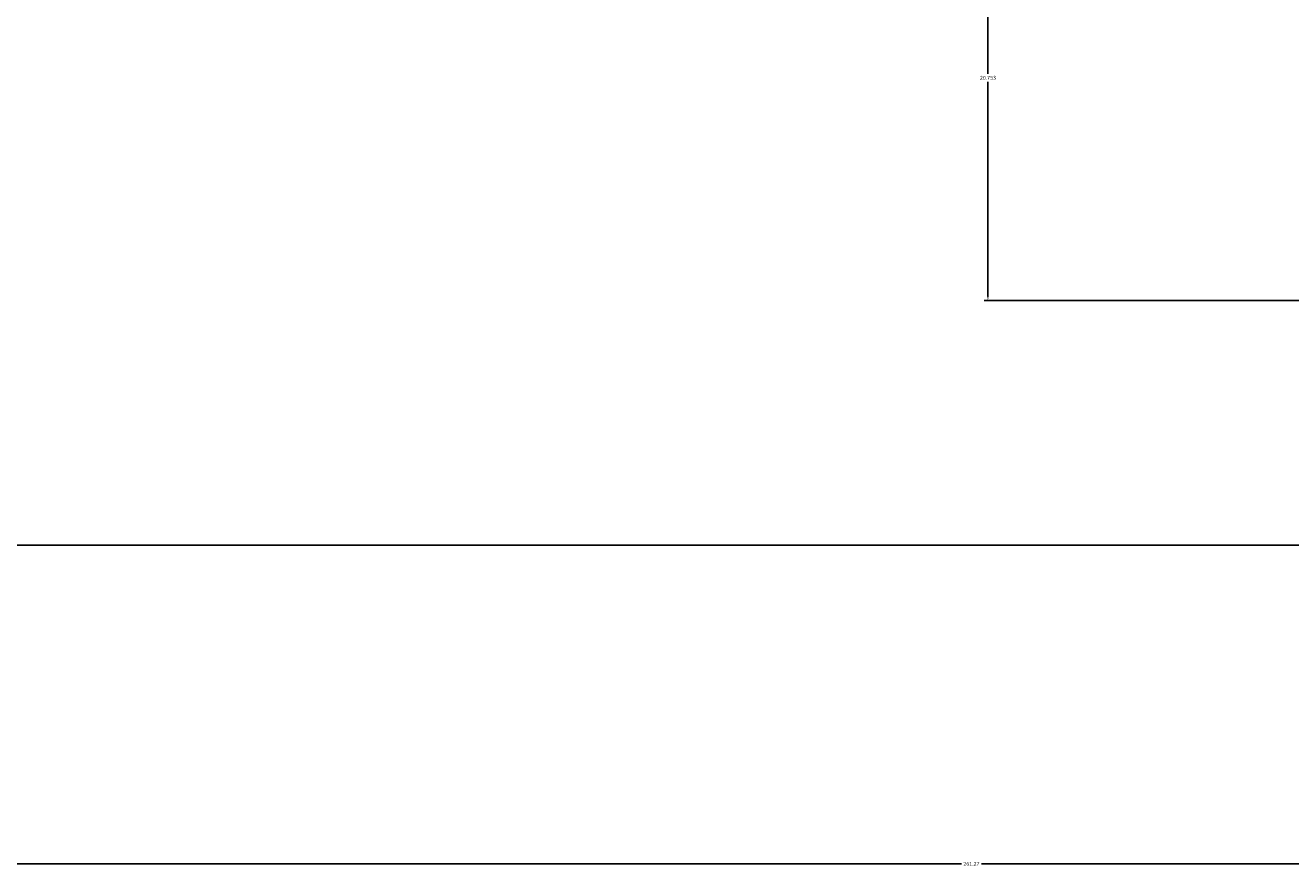
# Model space of a CAD drawing. Units: millimetres. Extents: x -11 to 280, y -4 to 208.
# Tile 19 of 55: x 91 to 150, y -4 to 36. Entities that reach past the tile are written whole.
import ezdxf

# ---------------------------------------------------------------- set-up
doc = ezdxf.new("R2010")
doc.units = ezdxf.units.MM
doc.layers.add('M-DIMS', color=2, linetype='Continuous', lineweight=18)
doc.styles.get("Standard").update_dxf_attribs({"font": 'arial.ttf'})
doc.dimstyles.get("Standard").update_dxf_attribs({"dimtxt": 0.18, "dimasz": 0.18, "dimexe": 0.18, "dimexo": 0.0625, "dimgap": 0.09, "dimtad": 0, "dimtih": 1, "dimtoh": 1, "dimdec": 4, "dimzin": 0, "dimdsep": 46, "dimtxsty": 'Standard', "dimcen": 0.09, "dimadec": 0, "dimazin": 0, "dimtfac": 1, "dimtdec": 4, "dimtofl": 0, "dimtmove": 0, "dimatfit": 3, "dimfxl": 1, "dimtolj": 1, "dimtzin": 0, "dimarcsym": 0})

# ---------------------------------------------------------------- blocks, each defined once
blk = doc.blocks.new('*D4')
at = {"layer": 'Defpoints', "color": 0, "transparency": 16777216}
for p in [(4.763, 84.426), (266.035, 51.733), (266.035, -3.415)]:
    blk.add_point(p, dxfattribs=at)
at = {"layer": 'M-DIMS', "color": 0, "lineweight": -2, "transparency": 16777216}
for p, q in [((4.763, 84.364), (4.763, -3.595)), ((266.035, 51.67), (266.035, -3.595)), ((4.943, -3.415), (134.934, -3.415)), ((265.855, -3.415), (135.864, -3.415))]:
    blk.add_line(p, q, dxfattribs=at)
at = {"layer": 'M-DIMS', "color": 0, "transparency": 16777216}
for points in [[(4.943, -3.385), (4.943, -3.445), (4.763, -3.415)], [(265.855, -3.385), (265.855, -3.445), (266.035, -3.415)]]:
    blk.add_solid(points, dxfattribs=at)
at = {"layer": 'M-DIMS', "color": 0, "transparency": 16777216, "insert": (135.399, -3.415), "char_height": 0.18, "attachment_point": 5}
blk.add_mtext('\\A1;261.27', dxfattribs=at)
blk = doc.blocks.new('*D5')
at = {"layer": 'Defpoints', "color": 0, "transparency": 16777216}
for p in [(24.759, 192.645), (-10.087, 11.435), (261.686, 11.435)]:
    blk.add_point(p, dxfattribs=at)
at = {"layer": 'M-DIMS', "color": 0, "lineweight": -2, "transparency": 16777216}
for p, q in [((24.696, 192.645), (-10.267, 192.645)), ((-10.087, 192.465), (-10.087, 102.222)), ((-10.087, 11.615), (-10.087, 101.858)), ((261.624, 11.435), (-10.267, 11.435))]:
    blk.add_line(p, q, dxfattribs=at)
at = {"layer": 'M-DIMS', "color": 0, "transparency": 16777216}
for points in [[(-10.117, 192.465), (-10.057, 192.465), (-10.087, 192.645)], [(-10.117, 11.615), (-10.057, 11.615), (-10.087, 11.435)]]:
    blk.add_solid(points, dxfattribs=at)
at = {"layer": 'M-DIMS', "color": 0, "transparency": 16777216, "insert": (-10.087, 102.04), "char_height": 0.18, "attachment_point": 5}
blk.add_mtext('\\A1;181.2', dxfattribs=at)
blk = doc.blocks.new('*D21')
at = {"layer": 'Defpoints', "color": 0, "transparency": 16777216}
for p in [(136.172, 43.599), (151.022, 43.599), (151.022, 22.846)]:
    blk.add_point(p, dxfattribs=at)
at = {"layer": 'M-DIMS', "color": 0, "lineweight": -2, "transparency": 16777216}
for p, q in [((150.959, 43.599), (135.992, 43.599)), ((136.172, 43.419), (136.172, 33.405)), ((136.172, 23.026), (136.172, 33.041)), ((150.959, 22.846), (135.992, 22.846))]:
    blk.add_line(p, q, dxfattribs=at)
at = {"layer": 'M-DIMS', "color": 0, "transparency": 16777216}
for points in [[(136.142, 43.419), (136.202, 43.419), (136.172, 43.599)], [(136.142, 23.026), (136.202, 23.026), (136.172, 22.846)]]:
    blk.add_solid(points, dxfattribs=at)
at = {"layer": 'M-DIMS', "color": 0, "transparency": 16777216, "insert": (136.172, 33.223), "char_height": 0.18, "attachment_point": 5}
blk.add_mtext('\\A1;20.753', dxfattribs=at)

msp = doc.modelspace()

# ---------------------------------------------------------------- dimensions: what is measured, and where the dimension line sits
at = {"layer": 'M-DIMS'}
for base, p1, p2, override, picture, middle in [((-10.0865, 11.4346), (24.7588, 192.645), (261.6863, 11.4346), {"dimdec": 1, "dimlfac": 1, "dimrnd": 0, "dimzin": 0, "dimdsep": 46, "dimlunit": 2}, '*D5', (-10.0865, 102.0398)), ((136.1717, 43.5991), (151.0217, 22.846), (151.0217, 43.5991), {"dimdec": 3, "dimlfac": 1, "dimrnd": 0, "dimzin": 0, "dimdsep": 46, "dimlunit": 2}, '*D21', (136.1717, 33.2226))]:
    dim = msp.add_linear_dim(base=base, p1=p1, p2=p2, angle=90, dimstyle='Standard', override=override, dxfattribs=at)
    dim.commit()
    dim.dimension.update_dxf_attribs({"geometry": picture, "text_midpoint": middle})
dim = msp.add_linear_dim(base=(266.0352, -3.4154), p1=(4.7635, 84.4261), p2=(266.0352, 51.7328), dimstyle='Standard', override={"dimdec": 2, "dimlfac": 1, "dimrnd": 0, "dimzin": 0, "dimdsep": 46, "dimlunit": 2}, dxfattribs=at)
dim.commit()
dim.dimension.update_dxf_attribs({"geometry": '*D4', "text_midpoint": (135.3993, -3.4154)})

doc.saveas('drawing.dxf')
